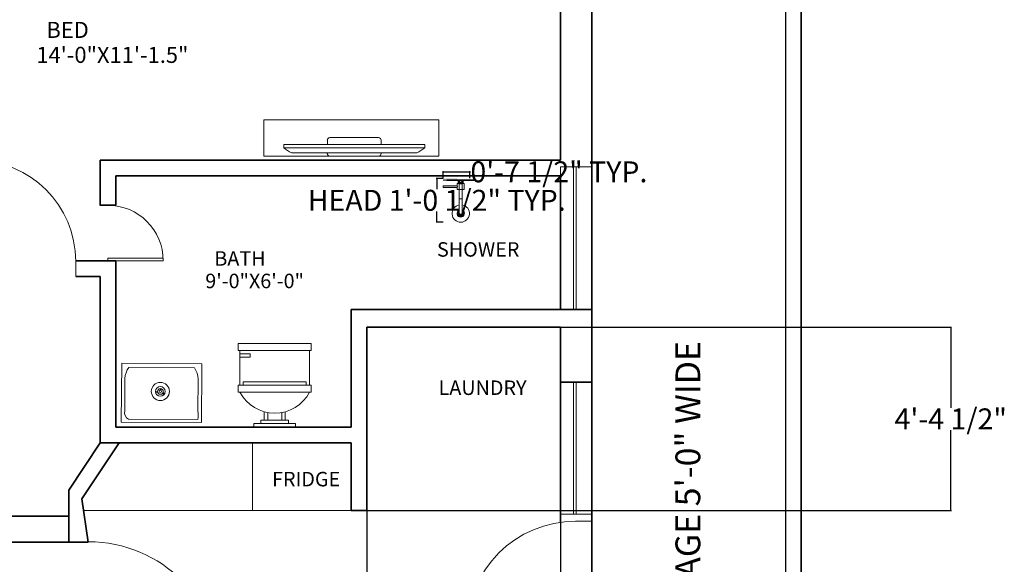
# Model space of a CAD drawing. Units: inches. Extents: x 79 to 8696167, y -3690578 to 147.
# Tile 6 of 10: x 329 to 612, y -223 to -67. Entities that reach past the tile are written whole.
import ezdxf

# ---------------------------------------------------------------- set-up
doc = ezdxf.new("R2010")
doc.units = ezdxf.units.IN
doc.header["$MEASUREMENT"] = 0
doc.layers.get('0').update_dxf_attribs({"color": 253})
for name, color, linetype, lineweight in [('A-ANNO-DIMS', 2, 'Continuous', 18), ('A-AREA-IDEN', 7, 'Continuous', 18), ('A-DOOR', 4, 'Continuous', 18), ('A-EQPM', 9, 'Continuous', 18), ('A-FLOR-CASE', 9, 'Continuous', 18), ('C-PROP', 7, 'Continuous', 35), ('C-SITE-WALL', 8, 'Continuous', 25), ('furniture', 30, 'Continuous', 18), ('PLUMBING FIXTURES', 9, 'Continuous', 18), ('walls', 8, 'Continuous', 35), ('windows', 171, 'Continuous', 18)]:
    doc.layers.add(name, color=color, linetype=linetype, lineweight=lineweight)
doc.styles.get("Standard").update_dxf_attribs({"font": 'arial.ttf'})
doc.dimstyles.get("Standard").update_dxf_attribs({"dimtxt": 6, "dimasz": 0.18, "dimexe": 0.18, "dimexo": 0.0625, "dimgap": 0.09, "dimtad": 0, "dimtih": 1, "dimtoh": 1, "dimzin": 0, "dimdsep": 46, "dimlunit": 3, "dimtxsty": 'Standard', "dimcen": 0.09, "dimadec": 0, "dimazin": 0, "dimtfac": 1, "dimtofl": 0, "dimtmove": 0, "dimatfit": 3, "dimfxl": 1, "dimtolj": 1, "dimtzin": 0, "dimarcsym": 0})

# ---------------------------------------------------------------- blocks, each defined once
blk = doc.blocks.new('PLASMA-LARGE')
at = {"layer": 'furniture'}
for p, q in [((-7.26, 0), (7.26, 0)), ((-21, -2.5), (21, -2.5)), ((-21, -2.5), (-21, -3.5)), ((-18.61, -1), (18.61, -1)), ((-8, -1), (-8, -0.74)), ((8, -1), (8, -0.74)), ((21, -2.5), (21, -3.5)), ((-21, -3.5), (21, -3.5)), ((-8, -3.5), (-8, -4.76)), ((-7.26, -5.5), (7.26, -5.5)), ((8, -3.5), (8, -4.76))]:
    blk.add_line(p, q, dxfattribs=at)
for centre, radius, start, end in [((-7.26, -0.74), 0.744, 90, 180), ((7.26, -0.74), 0.744, 0, 90), ((-13.97, -11.05), 11.07, 114.7602, 129.4175), ((13.97, -11.05), 11.07, 50.5825, 65.2398), ((-7.26, -4.76), 0.744, 180, 270), ((7.26, -4.76), 0.744, 270, 0)]:
    blk.add_arc(centre, radius, start, end, dxfattribs=at)
blk = doc.blocks.new('*U10')
for p, q in [((-10, 22), (-10, 12)), ((-10, 21), (-7, 21)), ((-7, 20), (-10, 20)), ((-7, 21), (-7, 20)), ((10, 12), (10, 22)), ((10.5, 12), (-10.5, 12)), ((-10.5, 10), (-10.5, 12)), ((9, 13), (-9, 13)), ((-9, 13), (-9, 12)), ((9, 12), (9, 13)), ((10.5, 12), (10.5, 10)), ((10.5, 10), (-10.5, 10)), ((-3, 4.4065), (-3, 2)), ((-2, 2), (-2, 4.1658)), ((2, 4.1658), (2, 2)), ((3, 2), (3, 4.4065)), ((4, 2), (-4, 2)), ((-4, 2), (-4, 1)), ((4, 1), (4, 2))]:
    blk.add_line(p, q)
for points in [[(10.5, 22), (10.5, 24), (-10.5, 24), (-10.5, 22)], [(6, 0), (6, 1), (-6, 1), (-6, 0)]]:
    blk.add_lwpolyline(points, close=True)
blk.add_arc((0, 15.3333), 11.3333, 208.0725, 331.9275)
blk = doc.blocks.new('O.H SHOWER-PL')
at = {"layer": 'PLUMBING FIXTURES'}
for points in [[(-1.84, 0), (-1.84, -0.25), (1.84, -0.25), (1.84, 0)], [(0.46, -8.72), (0.46, -9.67, -0.422337), (-0.46, -9.67), (-0.46, -8.72, 4.325472)]]:
    blk.add_hatch(color=256, dxfattribs=at).paths.add_polyline_path(points)
for p, q in [((-1.84, 0), (-1.84, -0.25)), ((1.84, 0), (-1.84, 0)), ((1.84, 0), (1.84, -0.25)), ((1.84, -0.25), (-1.84, -0.25)), ((-0.46, -0.25), (-0.46, -9.67)), ((0.46, -0.25), (0.46, -9.67))]:
    blk.add_line(p, q, dxfattribs=at)
for centre, radius, start, end in [((0, -4.48), 1.03, 243.53, 296.47), ((0, -9.67), 2.5, 100.61, 79.39), ((0, -9.67), 1.05, 116.0349, 63.9652), ((0, -9.22), 0.643, 224.2078, 315.7922)]:
    blk.add_arc(centre, radius, start, end, dxfattribs=at)
blk = doc.blocks.new('DIVERTER-PL')
at = {"layer": 'PLUMBING FIXTURES'}
for points in [[(4, 0), (-4, 0), (-4, -0.25), (4, -0.25)], [(0.38, -1.14), (0.38, -0.7), (-0.37, -0.7), (-0.37, -1.14)], [(1, -1.75, 0.30818), (1, -2.25), (5, -2.25), (5, -1.75)]]:
    blk.add_hatch(color=256, dxfattribs=at).paths.add_polyline_path(points)
for p, q in [((-4, 0), (-4, -0.25)), ((-4, 0), (4, 0)), ((4, 0), (4, -0.25)), ((-4, -0.25), (4, -0.25)), ((-4, -0.25), (4, -0.25)), ((-1, -1.05), (-0.37, -1.05)), ((-1, -1.05), (-1, -2.75)), ((-1, -2.75), (1, -2.75)), ((-0.75, -0.25), (-0.75, -1.05)), ((-0.37, -0.7), (0.38, -0.7)), ((-0.37, -0.7), (-0.37, -1.14)), ((-0.37, -1.14), (0.38, -1.14)), ((-0.32, -0.7), (-0.32, -0.25)), ((0.32, -0.7), (0.32, -0.25)), ((0.38, -0.7), (0.38, -1.14)), ((0.38, -1.05), (1, -1.05)), ((0.75, -0.25), (0.75, -1.05)), ((1, -1.05), (1, -1.75)), ((1, -2.25), (1, -2.75))]:
    blk.add_line(p, q, dxfattribs=at)
at = {"layer": 'PLUMBING FIXTURES', "ltscale": 12}
for p, q in [((1, -1.75), (5, -1.75)), ((1, -2.25), (5, -2.25)), ((5, -2.25), (5, -1.75))]:
    blk.add_line(p, q, dxfattribs=at)
at = {"layer": 'PLUMBING FIXTURES'}
blk.add_arc((1.37, -2), 0.444, 145.7435, 214.2565, dxfattribs=at)
blk = doc.blocks.new('A$C7F153053')
at = {"layer": 'PLUMBING FIXTURES', "xscale": -1, "rotation": 270}
for name in ['DIVERTER-PL', 'O.H SHOWER-PL']:
    blk.add_blockref(name, (12.17, 4), dxfattribs=at)
blk = doc.blocks.new('*U12')
for p, q in [((0, 0), (0, -6)), ((40, 0), (40, -6))]:
    blk.add_line(p, q)
blk.add_lwpolyline([(0, 0), (0, 40), (1.75, 40), (1.75, 0)], close=True)
blk.add_arc((0, 0), 40, 0, 90)
blk = doc.blocks.new('WIN-SIDE-41IN')
for p, q in [((0, 40.98), (9, 40.98)), ((0, 40.98), (0, 0)), ((3.73, 40.98), (3.73, 0)), ((4.5, 0), (4.5, 40.98)), ((9, 40.98), (9, 0)), ((9, 0), (0, 0))]:
    blk.add_line(p, q)
blk = doc.blocks.new('BASIN-RECT-DRAIN')
for p, q in [((0, 0.15), (0.11, 17)), ((0.11, 17), (23.11, 16.85)), ((20.97, 15.65), (2.15, 15.77)), ((23.1, 15.71), (23, 0)), ((23.11, 16.85), (23.1, 15.71)), ((0.99, 3.35), (1.05, 12.64)), ((21.96, 3.21), (22.03, 12.5)), ((10.4, 8.91), (9.84, 8.81)), ((10.52, 8.7), (9.87, 8.58)), ((11.22, 9.73), (11.16, 9.24)), ((11.36, 9.22), (11.4, 9.7)), ((11.97, 8.6), (12.36, 8.13)), ((11.84, 8.39), (12.22, 7.95)), ((23, 0), (0, 0.15)), ((21.95, 0.84), (2.06, 0.97))]:
    blk.add_line(p, q)
for radius in [2.61, 1.39, 0.816, 0.338]:
    blk.add_circle((11.22, 8.91), radius)
for centre, radius, start, end in [((6.46, 12.5), 5.4, 142.7525, 178.5493), ((16.62, 12.43), 5.4, 0.6949, 36.4918), ((3, 2.82), 2.08, 165.2338, 242.9258), ((12.7, 2.09), 9.33, 352.3124, 6.9318)]:
    blk.add_arc(centre, radius, start, end)
blk = doc.blocks.new('SHOWER-HEAD-DETAIL')
for points in [[(4, 12.56, -0.30818), (4, 12.06), (0, 12.06), (0, 12.56)], [(4, 12.56, -0.30818), (4, 12.06), (0, 12.06), (0, 12.56)], [(4, 12.56, -0.30818), (4, 12.06), (0, 12.06), (0, 12.56)], [(4, 12.56, -0.30818), (4, 12.06), (0, 12.06), (0, 12.56)], [(4, 12.56, -0.30818), (4, 12.06), (0, 12.06), (0, 12.56)], [(4, 12.56, -0.30818), (4, 12.06), (0, 12.06), (0, 12.56)], [(4, 12.56, -0.30818), (4, 12.06), (0, 12.06), (0, 12.56)], [(4, 12.56, -0.30818), (4, 12.06), (0, 12.06), (0, 12.56)], [(4, 12.56, -0.30818), (4, 12.06), (0, 12.06), (0, 12.56)], [(4, 12.56, -0.30818), (4, 12.06), (0, 12.06), (0, 12.56)], [(4, 12.56, -0.30818), (4, 12.06), (0, 12.06), (0, 12.56)], [(4, 12.56, -0.30818), (4, 12.06), (0, 12.06), (0, 12.56)], [(4, 12.56, -0.30818), (4, 12.06), (0, 12.06), (0, 12.56)], [(4, 12.56, -0.30818), (4, 12.06), (0, 12.06), (0, 12.56)], [(4, 12.56, -0.30818), (4, 12.06), (0, 12.06), (0, 12.56)], [(4, 12.56, -0.30818), (4, 12.06), (0, 12.06), (0, 12.56)], [(4, 12.56, -0.30818), (4, 12.06), (0, 12.06), (0, 12.56)], [(4, 12.56, -0.30818), (4, 12.06), (0, 12.06), (0, 12.56)], [(4, 12.56, -0.30818), (4, 12.06), (0, 12.06), (0, 12.56)], [(4, 12.56, -0.30818), (4, 12.06), (0, 12.06), (0, 12.56)], [(4, 12.56, -0.30818), (4, 12.06), (0, 12.06), (0, 12.56)], [(4, 12.56, -0.30818), (4, 12.06), (0, 12.06), (0, 12.56)], [(4, 12.56, -0.30818), (4, 12.06), (0, 12.06), (0, 12.56)], [(4, 12.56, -0.30818), (4, 12.06), (0, 12.06), (0, 12.56)], [(4, 12.56, -0.30818), (4, 12.06), (0, 12.06), (0, 12.56)], [(4, 12.56, -0.30818), (4, 12.06), (0, 12.06), (0, 12.56)], [(4, 12.56, -0.30818), (4, 12.06), (0, 12.06), (0, 12.56)], [(4, 12.56, -0.30818), (4, 12.06), (0, 12.06), (0, 12.56)], [(4, 12.56, -0.30818), (4, 12.06), (0, 12.06), (0, 12.56)], [(4, 12.56, -0.30818), (4, 12.06), (0, 12.06), (0, 12.56)], [(4, 12.56, -0.30818), (4, 12.06), (0, 12.06), (0, 12.56)], [(4, 12.56, -0.30818), (4, 12.06), (0, 12.06), (0, 12.56)], [(4, 12.56, -0.30818), (4, 12.06), (0, 12.06), (0, 12.56)], [(4, 12.56, -0.30818), (4, 12.06), (0, 12.06), (0, 12.56)], [(4, 12.56, -0.30818), (4, 12.06), (0, 12.06), (0, 12.56)], [(4, 12.56, -0.30818), (4, 12.06), (0, 12.06), (0, 12.56)], [(4.54, 3.44), (4.54, 2.5, 0.422337), (5.46, 2.5), (5.46, 3.44, -4.325472)], [(4.54, 3.44), (4.54, 2.5, 0.422337), (5.46, 2.5), (5.46, 3.44, -4.325472)], [(4.54, 3.44), (4.54, 2.5, 0.422337), (5.46, 2.5), (5.46, 3.44, -4.325472)], [(4.54, 3.44), (4.54, 2.5, 0.422337), (5.46, 2.5), (5.46, 3.44, -4.325472)], [(4.54, 3.44), (4.54, 2.5, 0.422337), (5.46, 2.5), (5.46, 3.44, -4.325472)], [(4.54, 3.44), (4.54, 2.5, 0.422337), (5.46, 2.5), (5.46, 3.44, -4.325472)], [(4.54, 3.44), (4.54, 2.5, 0.422337), (5.46, 2.5), (5.46, 3.44, -4.325472)], [(4.54, 3.44), (4.54, 2.5, 0.422337), (5.46, 2.5), (5.46, 3.44, -4.325472)], [(4.54, 3.44), (4.54, 2.5, 0.422337), (5.46, 2.5), (5.46, 3.44, -4.325472)], [(4.54, 3.44), (4.54, 2.5, 0.422337), (5.46, 2.5), (5.46, 3.44, -4.325472)], [(4.54, 3.44), (4.54, 2.5, 0.422337), (5.46, 2.5), (5.46, 3.44, -4.325472)], [(4.54, 3.44), (4.54, 2.5, 0.422337), (5.46, 2.5), (5.46, 3.44, -4.325472)], [(4.54, 3.44), (4.54, 2.5, 0.422337), (5.46, 2.5), (5.46, 3.44, -4.325472)], [(4.54, 3.44), (4.54, 2.5, 0.422337), (5.46, 2.5), (5.46, 3.44, -4.325472)], [(4.54, 3.44), (4.54, 2.5, 0.422337), (5.46, 2.5), (5.46, 3.44, -4.325472)], [(4.54, 3.44), (4.54, 2.5, 0.422337), (5.46, 2.5), (5.46, 3.44, -4.325472)], [(4.54, 3.44), (4.54, 2.5, 0.422337), (5.46, 2.5), (5.46, 3.44, -4.325472)], [(4.54, 3.44), (4.54, 2.5, 0.422337), (5.46, 2.5), (5.46, 3.44, -4.325472)], [(4.54, 3.44), (4.54, 2.5, 0.422337), (5.46, 2.5), (5.46, 3.44, -4.325472)], [(4.54, 3.44), (4.54, 2.5, 0.422337), (5.46, 2.5), (5.46, 3.44, -4.325472)], [(4.54, 3.44), (4.54, 2.5, 0.422337), (5.46, 2.5), (5.46, 3.44, -4.325472)], [(4.54, 3.44), (4.54, 2.5, 0.422337), (5.46, 2.5), (5.46, 3.44, -4.325472)], [(4.54, 3.44), (4.54, 2.5, 0.422337), (5.46, 2.5), (5.46, 3.44, -4.325472)], [(4.54, 3.44), (4.54, 2.5, 0.422337), (5.46, 2.5), (5.46, 3.44, -4.325472)], [(4.54, 3.44), (4.54, 2.5, 0.422337), (5.46, 2.5), (5.46, 3.44, -4.325472)], [(4.54, 3.44), (4.54, 2.5, 0.422337), (5.46, 2.5), (5.46, 3.44, -4.325472)], [(4.54, 3.44), (4.54, 2.5, 0.422337), (5.46, 2.5), (5.46, 3.44, -4.325472)], [(4.54, 3.44), (4.54, 2.5, 0.422337), (5.46, 2.5), (5.46, 3.44, -4.325472)], [(4.54, 3.44), (4.54, 2.5, 0.422337), (5.46, 2.5), (5.46, 3.44, -4.325472)], [(4.54, 3.44), (4.54, 2.5, 0.422337), (5.46, 2.5), (5.46, 3.44, -4.325472)], [(4.54, 3.44), (4.54, 2.5, 0.422337), (5.46, 2.5), (5.46, 3.44, -4.325472)], [(4.54, 3.44), (4.54, 2.5, 0.422337), (5.46, 2.5), (5.46, 3.44, -4.325472)], [(4.54, 3.44), (4.54, 2.5, 0.422337), (5.46, 2.5), (5.46, 3.44, -4.325472)], [(4.54, 3.44), (4.54, 2.5, 0.422337), (5.46, 2.5), (5.46, 3.44, -4.325472)], [(4.54, 3.44), (4.54, 2.5, 0.422337), (5.46, 2.5), (5.46, 3.44, -4.325472)], [(4.54, 3.44), (4.54, 2.5, 0.422337), (5.46, 2.5), (5.46, 3.44, -4.325472)], [(4.54, 3.44), (4.54, 2.5, 0.422337), (5.46, 2.5), (5.46, 3.44, -4.325472)], [(4.54, 3.44), (4.54, 2.5, 0.422337), (5.46, 2.5), (5.46, 3.44, -4.325472)]]:
    blk.add_hatch(color=256).paths.add_polyline_path(points)
at = {"ltscale": 12}
blk.add_line((4, 12.06), (0, 12.06), dxfattribs=at)
blk.add_line((4, 12.06), (0, 12.06), dxfattribs=at)
blk.add_line((4, 12.06), (0, 12.06), dxfattribs=at)
blk.add_line((4, 12.06), (0, 12.06), dxfattribs=at)
blk.add_line((4, 12.06), (0, 12.06), dxfattribs=at)
blk.add_line((4, 12.06), (0, 12.06), dxfattribs=at)
blk.add_line((4, 12.06), (0, 12.06), dxfattribs=at)
blk.add_line((4, 12.06), (0, 12.06), dxfattribs=at)
blk.add_line((4, 12.06), (0, 12.06), dxfattribs=at)
blk.add_line((4, 12.06), (0, 12.06), dxfattribs=at)
blk.add_line((4, 12.06), (0, 12.06), dxfattribs=at)
blk.add_line((4, 12.06), (0, 12.06), dxfattribs=at)
blk.add_line((4, 12.06), (0, 12.06), dxfattribs=at)
blk.add_line((4, 12.06), (0, 12.06), dxfattribs=at)
blk.add_line((4, 12.06), (0, 12.06), dxfattribs=at)
blk.add_line((4, 12.06), (0, 12.06), dxfattribs=at)
blk.add_line((4, 12.06), (0, 12.06), dxfattribs=at)
blk.add_line((4, 12.06), (0, 12.06), dxfattribs=at)
blk.add_line((4, 12.06), (0, 12.06), dxfattribs=at)
blk.add_line((4, 12.06), (0, 12.06), dxfattribs=at)
blk.add_line((4, 12.06), (0, 12.06), dxfattribs=at)
blk.add_line((4, 12.06), (0, 12.06), dxfattribs=at)
blk.add_line((4, 12.06), (0, 12.06), dxfattribs=at)
blk.add_line((4, 12.06), (0, 12.06), dxfattribs=at)
blk.add_line((4, 12.06), (0, 12.06), dxfattribs=at)
blk.add_line((4, 12.06), (0, 12.06), dxfattribs=at)
blk.add_line((4, 12.06), (0, 12.06), dxfattribs=at)
blk.add_line((4, 12.06), (0, 12.06), dxfattribs=at)
blk.add_line((4, 12.06), (0, 12.06), dxfattribs=at)
blk.add_line((4, 12.06), (0, 12.06), dxfattribs=at)
blk.add_line((4, 12.06), (0, 12.06), dxfattribs=at)
blk.add_line((4, 12.06), (0, 12.06), dxfattribs=at)
blk.add_line((4, 12.06), (0, 12.06), dxfattribs=at)
blk.add_line((4, 12.06), (0, 12.06), dxfattribs=at)
blk.add_line((4, 12.06), (0, 12.06), dxfattribs=at)
blk.add_line((4, 12.06), (0, 12.06), dxfattribs=at)
blk.add_line((4, 12.06), (0, 12.06), dxfattribs=at)
blk.add_line((4, 12.06), (0, 12.06), dxfattribs=at)
for p, q in [((4.54, 11.92), (4.54, 2.5)), ((4.54, 11.92), (4.54, 2.5)), ((4.54, 11.92), (4.54, 2.5)), ((4.54, 11.92), (4.54, 2.5)), ((4.54, 11.92), (4.54, 2.5)), ((4.54, 11.92), (4.54, 2.5)), ((4.54, 11.92), (4.54, 2.5)), ((4.54, 11.92), (4.54, 2.5)), ((4.54, 11.92), (4.54, 2.5)), ((4.54, 11.92), (4.54, 2.5)), ((4.54, 11.92), (4.54, 2.5)), ((4.54, 11.92), (4.54, 2.5)), ((4.54, 11.92), (4.54, 2.5)), ((4.54, 11.92), (4.54, 2.5)), ((4.54, 11.92), (4.54, 2.5)), ((4.54, 11.92), (4.54, 2.5)), ((4.54, 11.92), (4.54, 2.5)), ((4.54, 11.92), (4.54, 2.5)), ((4.54, 11.92), (4.54, 2.5)), ((4.54, 11.92), (4.54, 2.5)), ((4.54, 11.92), (4.54, 2.5)), ((4.54, 11.92), (4.54, 2.5)), ((4.54, 11.92), (4.54, 2.5)), ((4.54, 11.92), (4.54, 2.5)), ((4.54, 11.92), (4.54, 2.5)), ((4.54, 11.92), (4.54, 2.5)), ((4.54, 11.92), (4.54, 2.5)), ((4.54, 11.92), (4.54, 2.5)), ((4.54, 11.92), (4.54, 2.5)), ((4.54, 11.92), (4.54, 2.5)), ((4.54, 11.92), (4.54, 2.5)), ((4.54, 11.92), (4.54, 2.5)), ((4.54, 11.92), (4.54, 2.5)), ((4.54, 11.92), (4.54, 2.5)), ((4.54, 11.92), (4.54, 2.5)), ((4.54, 11.92), (4.54, 2.5)), ((4.54, 11.92), (4.54, 2.5)), ((4.54, 11.92), (4.54, 2.5)), ((5.46, 11.92), (5.46, 2.5)), ((5.46, 11.92), (5.46, 2.5)), ((5.46, 11.92), (5.46, 2.5)), ((5.46, 11.92), (5.46, 2.5)), ((5.46, 11.92), (5.46, 2.5)), ((5.46, 11.92), (5.46, 2.5)), ((5.46, 11.92), (5.46, 2.5)), ((5.46, 11.92), (5.46, 2.5)), ((5.46, 11.92), (5.46, 2.5)), ((5.46, 11.92), (5.46, 2.5)), ((5.46, 11.92), (5.46, 2.5)), ((5.46, 11.92), (5.46, 2.5)), ((5.46, 11.92), (5.46, 2.5)), ((5.46, 11.92), (5.46, 2.5)), ((5.46, 11.92), (5.46, 2.5)), ((5.46, 11.92), (5.46, 2.5)), ((5.46, 11.92), (5.46, 2.5)), ((5.46, 11.92), (5.46, 2.5)), ((5.46, 11.92), (5.46, 2.5)), ((5.46, 11.92), (5.46, 2.5)), ((5.46, 11.92), (5.46, 2.5)), ((5.46, 11.92), (5.46, 2.5)), ((5.46, 11.92), (5.46, 2.5)), ((5.46, 11.92), (5.46, 2.5)), ((5.46, 11.92), (5.46, 2.5)), ((5.46, 11.92), (5.46, 2.5)), ((5.46, 11.92), (5.46, 2.5)), ((5.46, 11.92), (5.46, 2.5)), ((5.46, 11.92), (5.46, 2.5)), ((5.46, 11.92), (5.46, 2.5)), ((5.46, 11.92), (5.46, 2.5)), ((5.46, 11.92), (5.46, 2.5)), ((5.46, 11.92), (5.46, 2.5)), ((5.46, 11.92), (5.46, 2.5)), ((5.46, 11.92), (5.46, 2.5)), ((5.46, 11.92), (5.46, 2.5)), ((5.46, 11.92), (5.46, 2.5)), ((5.46, 11.92), (5.46, 2.5))]:
    blk.add_line(p, q)
for centre, radius, start, end in [((5, 7.69), 1.03, 243.53, 296.47), ((5, 7.69), 1.03, 243.53, 296.47), ((5, 7.69), 1.03, 243.53, 296.47), ((5, 7.69), 1.03, 243.53, 296.47), ((5, 7.69), 1.03, 243.53, 296.47), ((5, 7.69), 1.03, 243.53, 296.47), ((5, 7.69), 1.03, 243.53, 296.47), ((5, 7.69), 1.03, 243.53, 296.47), ((5, 7.69), 1.03, 243.53, 296.47), ((5, 7.69), 1.03, 243.53, 296.47), ((5, 7.69), 1.03, 243.53, 296.47), ((5, 7.69), 1.03, 243.53, 296.47), ((5, 7.69), 1.03, 243.53, 296.47), ((5, 7.69), 1.03, 243.53, 296.47), ((5, 7.69), 1.03, 243.53, 296.47), ((5, 7.69), 1.03, 243.53, 296.47), ((5, 7.69), 1.03, 243.53, 296.47), ((5, 7.69), 1.03, 243.53, 296.47), ((5, 7.69), 1.03, 243.53, 296.47), ((5, 7.69), 1.03, 243.53, 296.47), ((5, 7.69), 1.03, 243.53, 296.47), ((5, 7.69), 1.03, 243.53, 296.47), ((5, 7.69), 1.03, 243.53, 296.47), ((5, 7.69), 1.03, 243.53, 296.47), ((5, 7.69), 1.03, 243.53, 296.47), ((5, 7.69), 1.03, 243.53, 296.47), ((5, 7.69), 1.03, 243.53, 296.47), ((5, 7.69), 1.03, 243.53, 296.47), ((5, 7.69), 1.03, 243.53, 296.47), ((5, 7.69), 1.03, 243.53, 296.47), ((5, 7.69), 1.03, 243.53, 296.47), ((5, 7.69), 1.03, 243.53, 296.47), ((5, 7.69), 1.03, 243.53, 296.47), ((5, 7.69), 1.03, 243.53, 296.47), ((5, 7.69), 1.03, 243.53, 296.47), ((5, 7.69), 1.03, 243.53, 296.47), ((5, 7.69), 1.03, 243.53, 296.47), ((5, 7.69), 1.03, 243.53, 296.47), ((5, 2.5), 2.5, 100.61, 79.39), ((5, 2.5), 2.5, 100.61, 79.39), ((5, 2.5), 2.5, 100.61, 79.39), ((5, 2.5), 2.5, 100.61, 79.39), ((5, 2.5), 2.5, 100.61, 79.39), ((5, 2.5), 2.5, 100.61, 79.39), ((5, 2.5), 2.5, 100.61, 79.39), ((5, 2.5), 2.5, 100.61, 79.39), ((5, 2.5), 2.5, 100.61, 79.39), ((5, 2.5), 2.5, 100.61, 79.39), ((5, 2.5), 2.5, 100.61, 79.39), ((5, 2.5), 2.5, 100.61, 79.39), ((5, 2.5), 2.5, 100.61, 79.39), ((5, 2.5), 2.5, 100.61, 79.39), ((5, 2.5), 2.5, 100.61, 79.39), ((5, 2.5), 2.5, 100.61, 79.39), ((5, 2.5), 2.5, 100.61, 79.39), ((5, 2.5), 2.5, 100.61, 79.39), ((5, 2.5), 2.5, 100.61, 79.39), ((5, 2.5), 2.5, 100.61, 79.39), ((5, 2.5), 2.5, 100.61, 79.39), ((5, 2.5), 2.5, 100.61, 79.39), ((5, 2.5), 2.5, 100.61, 79.39), ((5, 2.5), 2.5, 100.61, 79.39), ((5, 2.5), 2.5, 100.61, 79.39), ((5, 2.5), 2.5, 100.61, 79.39), ((5, 2.5), 2.5, 100.61, 79.39), ((5, 2.5), 2.5, 100.61, 79.39), ((5, 2.5), 2.5, 100.61, 79.39), ((5, 2.5), 2.5, 100.61, 79.39), ((5, 2.5), 2.5, 100.61, 79.39), ((5, 2.5), 2.5, 100.61, 79.39), ((5, 2.5), 2.5, 100.61, 79.39), ((5, 2.5), 2.5, 100.61, 79.39), ((5, 2.5), 2.5, 100.61, 79.39), ((5, 2.5), 2.5, 100.61, 79.39), ((5, 2.5), 2.5, 100.61, 79.39), ((5, 2.5), 2.5, 100.61, 79.39), ((5, 2.5), 1.05, 116.0348, 63.9651), ((5, 2.5), 1.05, 116.0348, 63.9651), ((5, 2.5), 1.05, 116.0348, 63.9651), ((5, 2.5), 1.05, 116.0348, 63.9651), ((5, 2.5), 1.05, 116.0348, 63.9651), ((5, 2.5), 1.05, 116.0348, 63.9651), ((5, 2.5), 1.05, 116.0348, 63.9651), ((5, 2.5), 1.05, 116.0348, 63.9651), ((5, 2.5), 1.05, 116.0348, 63.9651), ((5, 2.5), 1.05, 116.0348, 63.9651), ((5, 2.5), 1.05, 116.0348, 63.9651), ((5, 2.5), 1.05, 116.0348, 63.9651), ((5, 2.5), 1.05, 116.0348, 63.9651), ((5, 2.5), 1.05, 116.0348, 63.9651), ((5, 2.5), 1.05, 116.0348, 63.9651), ((5, 2.5), 1.05, 116.0348, 63.9651), ((5, 2.5), 1.05, 116.0348, 63.9651), ((5, 2.5), 1.05, 116.0348, 63.9651), ((5, 2.5), 1.05, 116.0348, 63.9651), ((5, 2.5), 1.05, 116.0348, 63.9651), ((5, 2.5), 1.05, 116.0348, 63.9651), ((5, 2.5), 1.05, 116.0348, 63.9651), ((5, 2.5), 1.05, 116.0348, 63.9651), ((5, 2.5), 1.05, 116.0348, 63.9651), ((5, 2.5), 1.05, 116.0348, 63.9651), ((5, 2.5), 1.05, 116.0348, 63.9651), ((5, 2.5), 1.05, 116.0348, 63.9651), ((5, 2.5), 1.05, 116.0348, 63.9651), ((5, 2.5), 1.05, 116.0348, 63.9651), ((5, 2.5), 1.05, 116.0348, 63.9651), ((5, 2.5), 1.05, 116.0348, 63.9651), ((5, 2.5), 1.05, 116.0348, 63.9651), ((5, 2.5), 1.05, 116.0348, 63.9651), ((5, 2.5), 1.05, 116.0348, 63.9651), ((5, 2.5), 1.05, 116.0348, 63.9651), ((5, 2.5), 1.05, 116.0348, 63.9651), ((5, 2.5), 1.05, 116.0348, 63.9651), ((5, 2.5), 1.05, 116.0348, 63.9651), ((5, 2.95), 0.643, 224.2078, 315.7922), ((5, 2.95), 0.643, 224.2078, 315.7922), ((5, 2.95), 0.643, 224.2078, 315.7922), ((5, 2.95), 0.643, 224.2078, 315.7922), ((5, 2.95), 0.643, 224.2078, 315.7922), ((5, 2.95), 0.643, 224.2078, 315.7922), ((5, 2.95), 0.643, 224.2078, 315.7922), ((5, 2.95), 0.643, 224.2078, 315.7922), ((5, 2.95), 0.643, 224.2078, 315.7922), ((5, 2.95), 0.643, 224.2078, 315.7922), ((5, 2.95), 0.643, 224.2078, 315.7922), ((5, 2.95), 0.643, 224.2078, 315.7922), ((5, 2.95), 0.643, 224.2078, 315.7922), ((5, 2.95), 0.643, 224.2078, 315.7922), ((5, 2.95), 0.643, 224.2078, 315.7922), ((5, 2.95), 0.643, 224.2078, 315.7922), ((5, 2.95), 0.643, 224.2078, 315.7922), ((5, 2.95), 0.643, 224.2078, 315.7922), ((5, 2.95), 0.643, 224.2078, 315.7922), ((5, 2.95), 0.643, 224.2078, 315.7922), ((5, 2.95), 0.643, 224.2078, 315.7922), ((5, 2.95), 0.643, 224.2078, 315.7922), ((5, 2.95), 0.643, 224.2078, 315.7922), ((5, 2.95), 0.643, 224.2078, 315.7922), ((5, 2.95), 0.643, 224.2078, 315.7922), ((5, 2.95), 0.643, 224.2078, 315.7922), ((5, 2.95), 0.643, 224.2078, 315.7922), ((5, 2.95), 0.643, 224.2078, 315.7922), ((5, 2.95), 0.643, 224.2078, 315.7922), ((5, 2.95), 0.643, 224.2078, 315.7922), ((5, 2.95), 0.643, 224.2078, 315.7922), ((5, 2.95), 0.643, 224.2078, 315.7922), ((5, 2.95), 0.643, 224.2078, 315.7922), ((5, 2.95), 0.643, 224.2078, 315.7922), ((5, 2.95), 0.643, 224.2078, 315.7922), ((5, 2.95), 0.643, 224.2078, 315.7922), ((5, 2.95), 0.643, 224.2078, 315.7922), ((5, 2.95), 0.643, 224.2078, 315.7922)]:
    blk.add_arc(centre, radius, start, end)
blk = doc.blocks.new('*D45')
at = {"layer": 'A-ANNO-DIMS', "color": 0, "lineweight": -2, "transparency": 16777216}
for p, q in [((450.76, -112.34), (448.76, -112.34)), ((448.94, -112.52), (448.94, -115.42)), ((448.94, -124.72), (448.94, -121.81)), ((450.76, -124.9), (448.76, -124.9))]:
    blk.add_line(p, q, dxfattribs=at)
at = {"layer": 'A-ANNO-DIMS', "color": 0, "lineweight": 100, "transparency": 16777216}
for points in [[(448.91, -112.52), (448.97, -112.52), (448.94, -112.34)], [(448.91, -124.72), (448.97, -124.72), (448.94, -124.9)]]:
    blk.add_solid(points, dxfattribs=at)
at = {"layer": 'Defpoints', "color": 0, "lineweight": 100, "transparency": 16777216}
for p in [(448.94, -112.34), (450.83, -112.34), (450.83, -124.9)]:
    blk.add_point(p, dxfattribs=at)
at = {"layer": 'A-ANNO-DIMS', "color": 0, "transparency": 16777216, "insert": (448.94, -118.62), "char_height": 6, "attachment_point": 5}
blk.add_mtext('\\A1;HEAD 1\'-0 1/2" TYP.', dxfattribs=at)
blk = doc.blocks.new('*D46')
at = {"layer": 'A-ANNO-DIMS', "color": 0, "lineweight": -2, "transparency": 16777216}
for p, q in [((450.83, -112.27), (450.83, -110.27)), ((451.01, -110.45), (458.26, -110.45)), ((458.44, -112.27), (458.44, -110.27)), ((458.44, -110.45), (458.62, -110.45))]:
    blk.add_line(p, q, dxfattribs=at)
at = {"layer": 'A-ANNO-DIMS', "color": 0, "lineweight": 100, "transparency": 16777216}
for points in [[(451.01, -110.42), (451.01, -110.48), (450.83, -110.45)], [(458.26, -110.42), (458.26, -110.48), (458.44, -110.45)]]:
    blk.add_solid(points, dxfattribs=at)
at = {"layer": 'Defpoints', "color": 0, "lineweight": 100, "transparency": 16777216}
for p in [(450.83, -112.34), (458.44, -110.45), (458.44, -112.34)]:
    blk.add_point(p, dxfattribs=at)
at = {"layer": 'A-ANNO-DIMS', "color": 0, "transparency": 16777216, "insert": (483.98, -110.45), "char_height": 6, "attachment_point": 5}
blk.add_mtext('\\A1;0\'-7 1/2" TYP.', dxfattribs=at)
blk = doc.blocks.new('*D57')
at = {"layer": 'A-ANNO-DIMS', "color": 0, "lineweight": -2, "transparency": 16777216}
for p, q in [((428.94, -155.06), (428.94, -723.2)), ((484.44, -155.06), (484.44, -723.2)), ((429.12, -723.02), (441.51, -723.02)), ((484.26, -723.02), (471.87, -723.02))]:
    blk.add_line(p, q, dxfattribs=at)
at = {"layer": 'A-ANNO-DIMS', "color": 0, "lineweight": 100, "transparency": 16777216}
for points in [[(429.12, -722.99), (429.12, -723.05), (428.94, -723.02)], [(484.26, -722.99), (484.26, -723.05), (484.44, -723.02)]]:
    blk.add_solid(points, dxfattribs=at)
at = {"layer": 'Defpoints', "color": 0, "lineweight": 100, "transparency": 16777216}
for p in [(428.94, -155), (484.44, -155), (484.44, -723.02)]:
    blk.add_point(p, dxfattribs=at)
at = {"layer": 'A-ANNO-DIMS', "color": 0, "transparency": 16777216, "insert": (456.69, -723.02), "char_height": 6, "attachment_point": 5}
blk.add_mtext('\\A1;4\'-7 1/2"', dxfattribs=at)
blk = doc.blocks.new('*D58')
at = {"layer": 'A-ANNO-DIMS', "color": 0, "lineweight": -2, "transparency": 16777216}
for p, q in [((429, -155), (596.52, -155)), ((596.34, -155.18), (596.34, -178.08)), ((596.34, -207.37), (596.34, -184.47)), ((429, -207.55), (596.52, -207.55))]:
    blk.add_line(p, q, dxfattribs=at)
at = {"layer": 'A-ANNO-DIMS', "color": 0, "lineweight": 100, "transparency": 16777216}
for points in [[(596.31, -155.18), (596.37, -155.18), (596.34, -155)], [(596.31, -207.37), (596.37, -207.37), (596.34, -207.55)]]:
    blk.add_solid(points, dxfattribs=at)
at = {"layer": 'Defpoints', "color": 0, "lineweight": 100, "transparency": 16777216}
for p in [(428.94, -155), (428.94, -207.55), (596.34, -207.55)]:
    blk.add_point(p, dxfattribs=at)
at = {"layer": 'A-ANNO-DIMS', "color": 0, "transparency": 16777216, "insert": (596.34, -181.27), "char_height": 6, "attachment_point": 5}
blk.add_mtext('\\A1;4\'-4 1/2"', dxfattribs=at)

msp = doc.modelspace()

# ---------------------------------------------------------------- linework, layer by layer
at = {"layer": 'A-EQPM'}
for p, q in [((396.165, -188.125), (396.165, -207.552)), ((424.441, -188.125), (396.165, -188.125)), ((424.441, -207.552), (424.441, -188.125)), ((396.165, -207.552), (424.441, -207.552))]:
    msp.add_line(p, q, dxfattribs=at)
at = {"layer": 'A-FLOR-CASE'}
for p, q in [((424.441, -207.552), (347.671, -207.552)), ((428.941, -207.552), (484.441, -207.552))]:
    msp.add_line(p, q, dxfattribs=at)
at = {"layer": 'C-PROP'}
msp.add_line((553.441, 99.875), (553.441, -680.125), dxfattribs=at)
at = {"layer": 'C-SITE-WALL'}
msp.add_line((548.941, 35.375), (548.941, -455.125), dxfattribs=at)
at = {"layer": 'furniture'}
msp.add_lwpolyline([(399.41, -95.582), (449.557, -95.582), (449.557, -105.954), (399.41, -105.954)], close=True, dxfattribs=at)
msp.add_lwpolyline([(399.41, -95.582), (449.557, -95.582), (449.557, -105.954), (399.41, -105.954)], close=True, dxfattribs=at)
at = {"layer": 'walls'}
for p, q in [((493.441, 35.375), (493.441, -455.125)), ((484.441, 26.375), (484.441, -107.125)), ((352.441, -107.125), (352.441, -120.035)), ((352.441, -107.125), (484.441, -107.125)), ((356.941, -111.625), (356.941, -120.035)), ((356.941, -111.625), (484.441, -111.625)), ((484.441, -111.625), (484.441, -149.875)), ((352.441, -120.035), (356.941, -120.035)), ((356.941, -135.921), (345.419, -135.921)), ((356.941, -140.446), (356.941, -135.921)), ((356.941, -135.921), (356.941, -183.625)), ((345.419, -140.446), (352.441, -140.446)), ((352.441, -140.446), (352.441, -188.125)), ((424.441, -149.875), (424.441, -183.625)), ((424.441, -149.875), (493.441, -149.875)), ((493.441, -170.759), (493.441, -149.875)), ((428.941, -154.996), (428.941, -188.125)), ((428.941, -154.996), (484.441, -154.996)), ((484.441, -154.996), (484.441, -170.759)), ((484.441, -154.996), (484.441, -210.901)), ((484.441, -170.759), (493.441, -170.759)), ((356.941, -183.625), (424.441, -183.625)), ((352.441, -188.125), (343.419, -201.7)), ((357.844, -188.125), (347.167, -204.191)), ((352.441, -188.125), (424.441, -188.125)), ((424.441, -207.552), (424.441, -188.125)), ((428.941, -207.552), (428.941, -188.125)), ((484.441, -188.125), (484.441, -210.901)), ((343.419, -201.7), (343.419, -216.625)), ((349.031, -216.625), (347.167, -204.191)), ((424.441, -207.552), (428.941, -207.552)), ((290.941, -209.184), (343.419, -209.184)), ((290.941, -216.625), (343.419, -216.625)), ((343.419, -216.625), (349.031, -216.625))]:
    msp.add_line(p, q, dxfattribs=at)
at = {"layer": 'windows'}
for p, q in [((484.441, -170.759), (493.441, -170.759)), ((484.441, -170.759), (484.441, -208.572)), ((488.168, -170.759), (488.168, -208.572)), ((488.941, -208.572), (488.941, -170.759)), ((493.441, -170.759), (493.441, -208.572)), ((493.441, -208.572), (484.441, -208.572))]:
    msp.add_line(p, q, dxfattribs=at)

# ---------------------------------------------------------------- block references
at = {"layer": 'A-DOOR', "xscale": 0.7244533731370114, "yscale": 0.7244533731370114, "zscale": 0.7244533731370114}
msp.add_blockref('*U12', (316.441, -136.099), dxfattribs=at)
at = {"layer": 'A-DOOR'}
for p, xscale, yscale, zscale, rotation in [((354.631, -135.921), -0.3973109503495726, 0.3973109503495726, 0.3973109503495726, 270), ((488.775, -241.705), 0.7776860473082563, 0.7776860473082563, 0.7776860473082563, 90), ((349.103, -254.372), -0.9472671488816434, 0.9472671488816434, 0.9472671488816434, 270)]:
    msp.add_blockref('*U12', p, dxfattribs=dict(at, xscale=xscale, yscale=yscale, zscale=zscale, rotation=rotation))
at = {"layer": 'furniture', "xscale": -0.9628364592350681, "yscale": 0.9628364592350692, "zscale": 0.9628364592350692, "rotation": 180.0045102986114}
msp.add_blockref('PLASMA-LARGE', (425.284, -105.954), dxfattribs=at)
msp.add_blockref('PLASMA-LARGE', (425.284, -105.954), dxfattribs=at)
at = {"layer": 'PLUMBING FIXTURES'}
for name, p in [('SHOWER-HEAD-DETAIL', (450.825, -124.896)), ('*U10', (402.491, -183.625)), ('BASIN-RECT-DRAIN', (358.495, -182.315))]:
    msp.add_blockref(name, p, dxfattribs=at)
at = {"layer": 'PLUMBING FIXTURES', "ltscale": 35, "rotation": 89.99999999999999}
msp.add_blockref('A$C7F153053', (459.825, -124.894), dxfattribs=at)
at = {"layer": 'windows'}
msp.add_blockref('WIN-SIDE-41IN', (484.441, -150.017), dxfattribs=at)

# ---------------------------------------------------------------- texts
at = {"layer": 'A-AREA-IDEN'}
for s, height, p in [('BED', 4.6103, (337.019, -72.077)), ('14\'-0"X11\'-1.5"', 4.61031, (334.135, -79.242)), ('SHOWER', 4.1556, (449.026, -134.773)), ('BATH', 4.1556, (385.181, -137.358)), ('9\'-0"X6\'-0"', 4.15558, (382.581, -143.815)), ('LAUNDRY', 4.1556, (449.474, -174.418)), ('FRIDGE', 4.1556, (401.737, -200.612))]:
    msp.add_text(s, height=height, dxfattribs=at).set_placement(p)
msp.add_text('PASSAGE 5\'-0" WIDE', height=7.11297, rotation=90, dxfattribs=at).set_placement((524.516, -250.409))

# ---------------------------------------------------------------- dimensions: what is measured, and where the dimension line sits
at = {"layer": 'A-ANNO-DIMS'}
dim = msp.add_linear_dim(base=(458.435, -110.451), p1=(450.825, -112.335), p2=(458.435, -112.335), text='<> TYP.', dimstyle='Standard', override={"dimdec": 1, "dimlfac": 1, "dimrnd": 0, "dimzin": 1, "dimdsep": 46, "dimlunit": 4, "dimfrac": 2}, dxfattribs=at)
dim.commit()
dim.dimension.update_dxf_attribs({"geometry": '*D46', "text_midpoint": (483.982, -110.451)})
dim = msp.add_linear_dim(base=(448.941, -112.335), p1=(450.825, -124.896), p2=(450.825, -112.335), angle=90, text='HEAD <> TYP.', dimstyle='Standard', override={"dimdec": 1, "dimlfac": 1, "dimrnd": 0, "dimzin": 1, "dimdsep": 46, "dimlunit": 4, "dimfrac": 2}, dxfattribs=at)
dim.commit()
dim.dimension.update_dxf_attribs({"geometry": '*D45', "text_midpoint": (448.941, -118.615)})
dim = msp.add_linear_dim(base=(484.441, -723.025), p1=(428.941, -154.996), p2=(484.441, -154.996), dimstyle='Standard', override={"dimdec": 1, "dimlfac": 1, "dimrnd": 0, "dimzin": 1, "dimdsep": 46, "dimlunit": 4, "dimfrac": 2}, dxfattribs=at)
dim.commit()
dim.dimension.update_dxf_attribs({"geometry": '*D57', "text_midpoint": (456.691, -723.025)})
dim = msp.add_linear_dim(base=(596.341, -207.552), p1=(428.941, -154.996), p2=(428.941, -207.552), angle=90, dimstyle='Standard', override={"dimdec": 1, "dimlfac": 1, "dimrnd": 0, "dimzin": 1, "dimdsep": 46, "dimlunit": 4, "dimfrac": 2}, dxfattribs=at)
dim.commit()
dim.dimension.update_dxf_attribs({"geometry": '*D58', "text_midpoint": (596.341, -181.274)})

doc.saveas('drawing.dxf')
